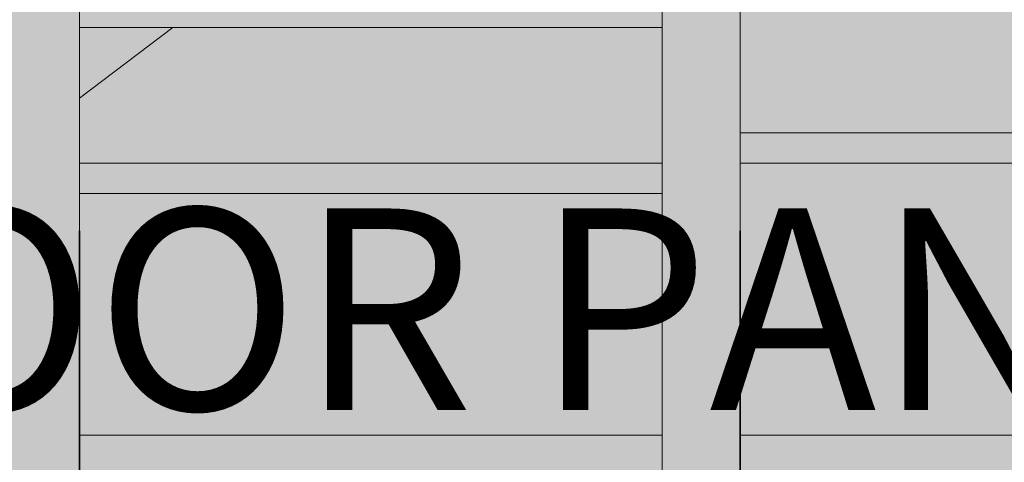
# Model space of a CAD drawing. Units: millimetres. Extents: x 130 to 1021, y 147 to 699.
# Tile 11 of 40: x 481 to 579, y 334 to 378. Entities that reach past the tile are written whole.
import ezdxf

# ---------------------------------------------------------------- set-up
doc = ezdxf.new("R2010")
doc.units = ezdxf.units.MM
doc.header["$MEASUREMENT"] = 0
for name, color, linetype, lineweight in [('A-ANNO-DIMS', 2, 'Continuous', 18), ('A-DOOR', 3, 'Continuous', 25), ('A-ELEV', 7, 'Continuous', 35), ('A-ELEV-PATT', 9, 'Continuous', 13), ('A-GLAZ', 4, 'Continuous', 18)]:
    doc.layers.add(name, color=color, linetype=linetype, lineweight=lineweight)
doc.styles.get("Standard").update_dxf_attribs({"font": 'arial.ttf'})
doc.dimstyles.get("Standard").update_dxf_attribs({"dimtxt": 20, "dimasz": 10, "dimexe": 10, "dimexo": 10, "dimgap": 5, "dimtad": 0, "dimtih": 1, "dimtoh": 1, "dimdec": 0, "dimzin": 0, "dimdsep": 46, "dimtxsty": 'Standard', "dimcen": 5, "dimadec": 0, "dimazin": 0, "dimtfac": 1, "dimtdec": 0, "dimtofl": 0, "dimtmove": 0, "dimatfit": 3, "dimfxl": 1, "dimtolj": 1, "dimtzin": 0, "dimarcsym": 0})

# ---------------------------------------------------------------- blocks, each defined once
blk = doc.blocks.new('*D7')
at = {"layer": 'A-ANNO-DIMS', "color": 0, "lineweight": -2, "transparency": 16777216}
for p, q in [((399.374, 349.447), (413.374, 349.447)), ((423.374, 349.447), (433.374, 349.447)), ((389.374, 344.547), (389.374, 339.447)), ((423.374, 344.547), (423.374, 339.447))]:
    blk.add_line(p, q, dxfattribs=at)
at = {"layer": 'A-ANNO-DIMS', "color": 0, "transparency": 16777216}
for points in [[(399.374, 351.114), (399.374, 347.781), (389.374, 349.447)], [(413.374, 351.114), (413.374, 347.781), (423.374, 349.447)]]:
    blk.add_solid(points, dxfattribs=at)
at = {"layer": 'Defpoints', "color": 0, "transparency": 16777216}
for p in [(389.374, 354.547), (423.374, 354.547), (423.374, 349.447)]:
    blk.add_point(p, dxfattribs=at)
at = {"layer": 'A-ANNO-DIMS', "color": 0, "transparency": 16777216, "insert": (582.037, 349.447), "char_height": 20, "attachment_point": 5}
blk.add_mtext('\\A1;DOOR PANEL 34 TYP.', dxfattribs=at)
blk = doc.blocks.new('*D8')
at = {"layer": 'A-ANNO-DIMS', "color": 0, "lineweight": -2, "transparency": 16777216}
for p, q in [((428.474, 380.947), (428.474, 390.947)), ((428.474, 390.947), (438.474, 390.947)), ((433.374, 370.947), (438.474, 370.947)), ((433.374, 354.547), (438.474, 354.547)), ((428.474, 344.547), (428.474, 334.547))]:
    blk.add_line(p, q, dxfattribs=at)
at = {"layer": 'A-ANNO-DIMS', "color": 0, "transparency": 16777216}
for points in [[(426.807, 380.947), (430.14, 380.947), (428.474, 370.947)], [(426.807, 344.547), (430.14, 344.547), (428.474, 354.547)]]:
    blk.add_solid(points, dxfattribs=at)
at = {"layer": 'Defpoints', "color": 0, "transparency": 16777216}
for p in [(423.374, 370.947), (428.474, 370.947), (423.374, 354.547)]:
    blk.add_point(p, dxfattribs=at)
at = {"layer": 'A-ANNO-DIMS', "color": 0, "transparency": 16777216, "insert": (491.209, 390.947), "char_height": 20, "attachment_point": 5}
blk.add_mtext('\\A1;16 TYP.', dxfattribs=at)
blk = doc.blocks.new('*D11')
at = {"layer": 'A-ANNO-DIMS', "color": 0, "lineweight": -2, "transparency": 16777216}
for p, q in [((737.374, 648.699), (737.374, 149.739)), ((299.374, 566.947), (299.374, 149.739)), ((309.374, 159.739), (490.857, 159.739)), ((727.374, 159.739), (545.891, 159.739))]:
    blk.add_line(p, q, dxfattribs=at)
at = {"layer": 'A-ANNO-DIMS', "color": 0, "transparency": 16777216}
for points in [[(309.374, 161.406), (309.374, 158.073), (299.374, 159.739)], [(727.374, 161.406), (727.374, 158.073), (737.374, 159.739)]]:
    blk.add_solid(points, dxfattribs=at)
at = {"layer": 'Defpoints', "color": 0, "transparency": 16777216}
for p in [(737.374, 658.699), (299.374, 576.947), (737.374, 159.739)]:
    blk.add_point(p, dxfattribs=at)
at = {"layer": 'A-ANNO-DIMS', "color": 0, "transparency": 16777216, "insert": (518.374, 159.739), "char_height": 20, "attachment_point": 5}
blk.add_mtext('\\A1;438', dxfattribs=at)
blk = doc.blocks.new('*D12')
at = {"layer": 'A-ANNO-DIMS', "color": 0, "lineweight": -2, "transparency": 16777216}
for p, q in [((477.374, 661.947), (265.074, 661.947)), ((275.074, 651.947), (275.074, 438.205)), ((275.074, 194.039), (275.074, 407.782)), ((357.163, 184.039), (265.074, 184.039))]:
    blk.add_line(p, q, dxfattribs=at)
at = {"layer": 'A-ANNO-DIMS', "color": 0, "transparency": 16777216}
for points in [[(273.407, 651.947), (276.74, 651.947), (275.074, 661.947)], [(273.407, 194.039), (276.74, 194.039), (275.074, 184.039)]]:
    blk.add_solid(points, dxfattribs=at)
at = {"layer": 'Defpoints', "color": 0, "transparency": 16777216}
for p in [(275.074, 661.947), (487.374, 661.947), (367.163, 184.039)]:
    blk.add_point(p, dxfattribs=at)
at = {"layer": 'A-ANNO-DIMS', "color": 0, "transparency": 16777216, "insert": (275.074, 422.993), "char_height": 20, "attachment_point": 5}
blk.add_mtext('\\A1;477.9', dxfattribs=at)
blk = doc.blocks.new('*D23')
at = {"layer": 'A-ANNO-DIMS', "color": 0, "lineweight": -2, "transparency": 16777216}
for p, q in [((466.767, 403.947), (466.767, 696.247)), ((475.988, 209.039), (475.988, 696.247)), ((456.767, 686.247), (446.767, 686.247)), ((485.988, 686.247), (495.988, 686.247))]:
    blk.add_line(p, q, dxfattribs=at)
at = {"layer": 'A-ANNO-DIMS', "color": 0, "transparency": 16777216}
for points in [[(456.767, 687.914), (456.767, 684.581), (466.767, 686.247)], [(485.988, 687.914), (485.988, 684.581), (475.988, 686.247)]]:
    blk.add_solid(points, dxfattribs=at)
at = {"layer": 'Defpoints', "color": 0, "transparency": 16777216}
for p in [(475.988, 686.247), (466.767, 393.947), (475.988, 199.039)]:
    blk.add_point(p, dxfattribs=at)
at = {"layer": 'A-ANNO-DIMS', "color": 0, "transparency": 16777216, "insert": (534.631, 686.247), "char_height": 20, "attachment_point": 5}
blk.add_mtext('\\A1;9.222', dxfattribs=at)
blk = doc.blocks.new('*D24')
at = {"layer": 'A-ANNO-DIMS', "color": 0, "lineweight": -2, "transparency": 16777216}
for p, q in [((475.988, 209.039), (475.988, 696.247)), ((487.374, 671.947), (487.374, 696.247)), ((465.988, 686.247), (455.988, 686.247)), ((497.374, 686.247), (507.374, 686.247))]:
    blk.add_line(p, q, dxfattribs=at)
at = {"layer": 'A-ANNO-DIMS', "color": 0, "transparency": 16777216}
for points in [[(465.988, 687.914), (465.988, 684.581), (475.988, 686.247)], [(497.374, 687.914), (497.374, 684.581), (487.374, 686.247)]]:
    blk.add_solid(points, dxfattribs=at)
at = {"layer": 'Defpoints', "color": 0, "transparency": 16777216}
for p in [(487.374, 686.247), (487.374, 661.947), (475.988, 199.039)]:
    blk.add_point(p, dxfattribs=at)
at = {"layer": 'A-ANNO-DIMS', "color": 0, "transparency": 16777216, "insert": (553.022, 686.247), "char_height": 20, "attachment_point": 5}
blk.add_mtext('\\A1;11.385', dxfattribs=at)
blk = doc.blocks.new('*D51')
at = {"layer": 'A-ANNO-DIMS', "color": 0, "lineweight": -2, "transparency": 16777216}
for p, q in [((554.635, 386.264), (771.674, 386.264)), ((761.674, 376.264), (761.674, 348.674)), ((761.674, 290.662), (761.674, 318.251)), ((554.635, 280.662), (771.674, 280.662))]:
    blk.add_line(p, q, dxfattribs=at)
at = {"layer": 'A-ANNO-DIMS', "color": 0, "transparency": 16777216}
for points in [[(760.007, 376.264), (763.34, 376.264), (761.674, 386.264)], [(760.007, 290.662), (763.34, 290.662), (761.674, 280.662)]]:
    blk.add_solid(points, dxfattribs=at)
at = {"layer": 'Defpoints', "color": 0, "transparency": 16777216}
for p in [(544.635, 386.264), (761.674, 386.264), (544.635, 280.662)]:
    blk.add_point(p, dxfattribs=at)
at = {"layer": 'A-ANNO-DIMS', "color": 0, "transparency": 16777216, "insert": (761.674, 333.463), "char_height": 20, "attachment_point": 5}
blk.add_mtext('\\A1;105.6', dxfattribs=at)
blk = doc.blocks.new('*D52')
at = {"layer": 'A-ANNO-DIMS', "color": 0, "lineweight": -2, "transparency": 16777216}
for p, q in [((761.674, 403.947), (761.674, 413.947)), ((761.674, 413.947), (771.674, 413.947)), ((642.818, 393.947), (771.674, 393.947)), ((554.635, 386.264), (771.674, 386.264)), ((761.674, 376.264), (761.674, 366.264))]:
    blk.add_line(p, q, dxfattribs=at)
at = {"layer": 'A-ANNO-DIMS', "color": 0, "transparency": 16777216}
for points in [[(760.007, 403.947), (763.34, 403.947), (761.674, 393.947)], [(760.007, 376.264), (763.34, 376.264), (761.674, 386.264)]]:
    blk.add_solid(points, dxfattribs=at)
at = {"layer": 'Defpoints', "color": 0, "transparency": 16777216}
for p in [(632.818, 393.947), (761.674, 393.947), (544.635, 386.264)]:
    blk.add_point(p, dxfattribs=at)
at = {"layer": 'A-ANNO-DIMS', "color": 0, "transparency": 16777216, "insert": (810.337, 413.947), "char_height": 20, "attachment_point": 5}
blk.add_mtext('\\A1;7.683', dxfattribs=at)
blk = doc.blocks.new('*D64')
at = {"layer": 'A-ANNO-DIMS', "color": 0, "lineweight": -2, "transparency": 16777216}
for p, q in [((502.049, 450.926), (502.049, 460.926)), ((497.049, 455.926), (507.049, 455.926)), ((363.96, 263.061), (409.922, 327.255)), ((353.96, 263.061), (363.96, 263.061))]:
    blk.add_line(p, q, dxfattribs=at)
at = {"layer": 'A-ANNO-DIMS', "color": 0, "transparency": 16777216}
blk.add_solid([(408.567, 328.225), (411.277, 326.284), (415.743, 335.385)], dxfattribs=at)
at = {"layer": 'Defpoints', "color": 0, "transparency": 16777216}
for p in [(502.049, 455.926), (415.743, 335.385)]:
    blk.add_point(p, dxfattribs=at)
at = {"layer": 'A-ANNO-DIMS', "color": 0, "transparency": 16777216, "insert": (297.8, 263.061), "char_height": 20, "attachment_point": 5}
blk.add_mtext('\\A1;R148.25', dxfattribs=at)
blk = doc.blocks.new('*D65')
at = {"layer": 'A-ANNO-DIMS', "color": 0, "lineweight": -2, "transparency": 16777216}
for p, q in [((495.463, 509.127), (472.508, 423.108)), ((505.463, 509.127), (495.463, 509.127)), ((427.374, 248.979), (427.374, 258.979)), ((422.374, 253.979), (432.374, 253.979))]:
    blk.add_line(p, q, dxfattribs=at)
at = {"layer": 'A-ANNO-DIMS', "color": 0, "transparency": 16777216}
blk.add_solid([(470.898, 423.538), (474.118, 422.679), (469.93, 413.447)], dxfattribs=at)
at = {"layer": 'Defpoints', "color": 0, "transparency": 16777216}
for p in [(469.93, 413.447), (427.374, 253.979)]:
    blk.add_point(p, dxfattribs=at)
at = {"layer": 'A-ANNO-DIMS', "color": 0, "transparency": 16777216, "insert": (561.623, 509.127), "char_height": 20, "attachment_point": 5}
blk.add_mtext('\\A1;R165.05', dxfattribs=at)
blk = doc.blocks.new('*D67')
at = {"layer": 'A-ANNO-DIMS', "color": 0, "lineweight": -2, "transparency": 16777216}
for p, q in [((479.756, 492.431), (462.144, 412.223)), ((489.756, 492.431), (479.756, 492.431)), ((427.07, 247.496), (427.07, 257.496)), ((422.07, 252.496), (432.07, 252.496))]:
    blk.add_line(p, q, dxfattribs=at)
at = {"layer": 'A-ANNO-DIMS', "color": 0, "transparency": 16777216}
blk.add_solid([(460.516, 412.58), (463.772, 411.865), (459.999, 402.455)], dxfattribs=at)
at = {"layer": 'Defpoints', "color": 0, "transparency": 16777216}
for p in [(459.999, 402.455), (427.07, 252.496)]:
    blk.add_point(p, dxfattribs=at)
at = {"layer": 'A-ANNO-DIMS', "color": 0, "transparency": 16777216, "insert": (545.841, 492.431), "char_height": 20, "attachment_point": 5}
blk.add_mtext('\\A1;R153.53', dxfattribs=at)
blk = doc.blocks.new('*D69')
at = {"layer": 'A-ANNO-DIMS', "color": 0, "lineweight": -2, "transparency": 16777216}
for p, q in [((507.746, 572.261), (483.091, 501.813)), ((517.746, 572.261), (507.746, 572.261)), ((433.191, 354.23), (433.191, 364.23)), ((428.191, 359.23), (438.191, 359.23))]:
    blk.add_line(p, q, dxfattribs=at)
at = {"layer": 'A-ANNO-DIMS', "color": 0, "transparency": 16777216}
blk.add_solid([(481.518, 502.363), (484.664, 501.262), (479.788, 492.374)], dxfattribs=at)
at = {"layer": 'Defpoints', "color": 0, "transparency": 16777216}
for p in [(479.788, 492.374), (433.191, 359.23)]:
    blk.add_point(p, dxfattribs=at)
at = {"layer": 'A-ANNO-DIMS', "color": 0, "transparency": 16777216, "insert": (573.824, 572.261), "char_height": 20, "attachment_point": 5}
blk.add_mtext('\\A1;R141.06', dxfattribs=at)
blk = doc.blocks.new('*D71')
at = {"layer": 'A-ANNO-DIMS', "color": 0, "lineweight": -2, "transparency": 16777216}
for p, q in [((492.108, 581.609), (472.542, 512.666)), ((502.108, 581.609), (492.108, 581.609)), ((432.65, 367.109), (432.65, 377.109)), ((427.65, 372.109), (437.65, 372.109))]:
    blk.add_line(p, q, dxfattribs=at)
at = {"layer": 'A-ANNO-DIMS', "color": 0, "transparency": 16777216}
blk.add_solid([(470.938, 513.121), (474.145, 512.211), (469.812, 503.046)], dxfattribs=at)
at = {"layer": 'Defpoints', "color": 0, "transparency": 16777216}
for p in [(469.812, 503.046), (432.65, 372.109)]:
    blk.add_point(p, dxfattribs=at)
at = {"layer": 'A-ANNO-DIMS', "color": 0, "transparency": 16777216, "insert": (548.493, 581.609), "char_height": 20, "attachment_point": 5}
blk.add_mtext('\\A1;R136.1', dxfattribs=at)
blk = doc.blocks.new('*D72')
at = {"layer": 'A-ANNO-DIMS', "color": 0, "lineweight": -2, "transparency": 16777216}
for p, q in [((460.658, 573.64), (451.279, 503.49)), ((470.658, 573.64), (460.658, 573.64)), ((432.115, 355.142), (432.115, 365.142)), ((427.115, 360.142), (437.115, 360.142))]:
    blk.add_line(p, q, dxfattribs=at)
at = {"layer": 'A-ANNO-DIMS', "color": 0, "transparency": 16777216}
blk.add_solid([(449.628, 503.711), (452.931, 503.27), (449.954, 493.579)], dxfattribs=at)
at = {"layer": 'Defpoints', "color": 0, "transparency": 16777216}
for p in [(449.954, 493.579), (432.115, 360.142)]:
    blk.add_point(p, dxfattribs=at)
at = {"layer": 'A-ANNO-DIMS', "color": 0, "transparency": 16777216, "insert": (526.64, 573.64), "char_height": 20, "attachment_point": 5}
blk.add_mtext('\\A1;R134.62', dxfattribs=at)

msp = doc.modelspace()

# ---------------------------------------------------------------- hatches: boundary and pattern name
at = {"layer": 'A-ELEV-PATT'}
h = msp.add_hatch(color=256, dxfattribs=at)
h.dxf.hatch_style = 1
h.paths.add_polyline_path([(737.3738, 658.6988, 0.0135961), (632.4019, 661.9473), (607.3738, 661.9473), (487.3738, 661.9473), (487.3738, 649.9473), (607.3738, 649.9473), (632.3794, 649.9473, -0.0136841), (737.3738, 646.6784)])
h.paths.add_polyline_path([(732.3738, 643.9599, 0.0130529), (632.3738, 646.9473), (607.3738, 646.9473), (487.3738, 646.9473), (487.3738, 596.9473), (632.3738, 596.9473, -0.0130529), (732.3738, 593.9599)])
h.paths.add_polyline_path([(737.3738, 593.6732, 0.0137063), (632.3738, 596.9473), (487.3738, 596.9473), (487.3738, 586.9473), (632.355, 586.9473, -0.0137808), (737.3738, 583.6559)])
h.paths.add_polyline_path([(447.3738, 646.9473), (307.3738, 646.9473), (302.3738, 646.9473), (302.3738, 634.9473), (447.3738, 634.9473)])
h.paths.add_polyline_path([(447.3738, 631.9473), (307.3738, 631.9473), (307.3738, 586.9473), (447.3738, 586.9473)])
h.paths.add_polyline_path([(447.3738, 586.9473), (307.3738, 586.9473), (302.3738, 586.9473), (302.3738, 576.9473), (447.3738, 576.9473)])
h.paths.add_polyline_path([(447.3738, 573.9473), (367.3738, 573.9473), (367.3738, 539.9473), (447.3738, 539.9473)])
h.paths.add_polyline_path([(447.3738, 537.9473), (367.3738, 537.9473), (367.3738, 507.9473), (400.392, 507.4253, -0.001728), (401.3281, 507.6451, -0.5220025), (425.6117, 511.0391, -0.0391849), (447.3738, 510.4359), (447.3738, 510.7883)])
h.paths.add_polyline_path([(394.7238, 505.9473), (367.3738, 505.9473), (367.3738, 476.9473, -0.0146512), (375.8501, 480.2159), (376.1506, 499.2266, -0.0355419)])
h.paths.add_polyline_path([(632.3738, 583.9473), (552.3738, 583.9473), (552.3738, 550.9473), (632.3738, 550.9473)])
h.paths.add_polyline_path([(632.3738, 548.9473), (552.3738, 548.9473), (552.3738, 515.9473), (632.3738, 515.9473)])
h.paths.add_polyline_path([(632.3738, 513.9473), (552.3738, 513.9473), (552.3738, 476.9473), (632.3738, 476.9473)])
h.paths.add_polyline_path([(737.3738, 473.6903, 0.0136326), (632.3926, 476.9473), (552.3738, 476.9473), (487.3738, 476.9473), (487.3738, 466.9473), (632.3738, 466.9473, -0.0137063), (737.3738, 463.6732)])
h.paths.add_polyline_path([(732.3738, 460.9552, 0.0130741), (632.3681, 463.9473), (487.3738, 463.9473), (487.3738, 407.735, -0.0032286), (489.3544, 406.9473), (632.3926, 406.9473, -0.0129826), (732.3738, 403.9755)])
h.paths.add_polyline_path([(487.3738, 463.9473, 0.20133), (367.3738, 463.9473), (367.3738, 407.735, -0.1882031), (487.3738, 407.735)])
h.paths.add_polyline_path([(367.3738, 476.9473), (367.3738, 466.9473, -0.2013309), (487.3738, 466.9473), (487.3738, 476.9473, 0.20133)])
h.paths.add_polyline_path([(367.3738, 463.9473), (307.3738, 463.9473), (307.3738, 401.9473), (357.9413, 401.9473), (367.3738, 407.735)])
h.paths.add_polyline_path([(367.3738, 476.9473), (302.3738, 476.9473), (302.3738, 466.9473), (367.3738, 466.9473)])
h.paths.add_polyline_path([(632.8184, 366.9453), (552.3738, 366.9453), (552.3738, 393.9473), (632.8184, 393.9473)])
h.paths.add_polyline_path([(632.8184, 357.2114), (632.8184, 363.9453), (552.3738, 363.9453), (552.3738, 357.2114), (552.3738, 336.9453), (632.8184, 336.9453)])
h.paths.add_polyline_path([(632.8184, 333.9453), (552.3738, 333.9453), (552.3738, 306.9453), (632.8184, 306.9453)])
h.paths.add_polyline_path([(632.8184, 303.9453), (552.3738, 303.9453), (552.3738, 273.9473), (632.355, 273.9473, 0.0000608), (632.8184, 273.9491)])
h.paths.add_polyline_path([(737.3738, 403.6903, 0.0136326), (632.3926, 406.9473), (489.3544, 406.9473, 0.1915481), (367.3738, 407.735), (367.3738, 396.9473, -0.2013309), (487.3738, 396.9473), (632.3738, 396.9473, -0.0137063), (737.3738, 393.6732)])
h.paths.add_polyline_path([(357.9413, 401.9473), (307.3738, 401.9473), (307.3738, 391.9473), (357.9413, 391.9473)])
h.paths.add_polyline_path([(357.9413, 357.2114), (357.9413, 388.9473), (307.3738, 388.9473), (307.3738, 357.2114), (307.3738, 273.9473), (357.9413, 273.9473)])
h.paths.add_polyline_path([(732.3738, 263.93, -0.0130317), (632.3794, 260.9473), (466.7667, 260.9473), (466.7667, 240.9473), (469.8406, 236.978), (469.8406, 221.978), (472.9145, 218.0087), (472.9145, 213.9473), (607.3738, 213.9473), (732.3738, 213.9473)])
h.paths.add_polyline_path([(732.3738, 290.889), (722.479, 290.889), (722.479, 301.889), (732.3738, 301.889), (732.3738, 305.889), (722.479, 305.889), (722.479, 316.889), (732.3738, 316.889), (732.3738, 320.889), (722.479, 320.889), (722.479, 331.889), (732.3738, 331.889), (732.3738, 335.889), (722.479, 335.889), (722.479, 346.889), (732.3738, 346.889), (732.3738, 350.889), (722.479, 350.889), (722.479, 361.889), (732.3738, 361.889), (732.3738, 365.889), (722.479, 365.889), (722.479, 376.889), (732.3738, 376.889), (732.3738, 380.889), (722.479, 380.889), (722.479, 391.4848, 0.0005233), (718.479, 391.6843), (718.479, 380.889), (707.479, 380.889), (707.479, 392.1896, 0.0005231), (703.479, 392.3576), (703.479, 380.889), (692.479, 380.889), (692.479, 392.7765, 0.0005229), (688.479, 392.9131), (688.479, 380.889), (677.479, 380.889), (677.479, 393.2456, 0.0005228), (673.479, 393.3508), (673.479, 380.889), (662.479, 380.889), (662.479, 393.597, 0.0005227), (658.479, 393.6709), (658.479, 380.889), (647.479, 380.889), (647.479, 393.8308, 0.0005226), (643.479, 393.8732), (643.479, 380.889), (632.8184, 380.889), (632.8184, 376.889), (643.479, 376.889), (643.479, 365.889), (632.8184, 365.889), (632.8184, 361.889), (643.479, 361.889), (643.479, 350.889), (632.8184, 350.889), (632.8184, 346.889), (643.479, 346.889), (643.479, 335.889), (632.8184, 335.889), (632.8184, 331.889), (643.479, 331.889), (643.479, 320.889), (632.8184, 320.889), (632.8184, 316.889), (643.479, 316.889), (643.479, 305.889), (632.8184, 305.889), (632.8184, 301.889), (643.479, 301.889), (643.479, 290.889), (632.8184, 290.889), (632.8184, 286.889), (643.479, 286.889), (643.479, 274.0217, 0.0005246), (647.479, 274.0643), (647.479, 286.889), (658.479, 286.889), (658.479, 274.2248, 0.0005246), (662.479, 274.2989), (662.479, 286.889), (673.479, 286.889), (673.479, 274.546, 0.0005247), (677.479, 274.6516), (677.479, 286.889), (688.479, 286.889), (688.479, 274.9853, 0.0005248), (692.479, 275.1224), (692.479, 286.889), (703.479, 286.889), (703.479, 275.5429, 0.000525), (707.479, 275.7115), (707.479, 286.889), (718.479, 286.889), (718.479, 276.2187, 0.0005252), (722.479, 276.4189), (722.479, 286.889), (732.3738, 286.889)])
h.paths.add_polyline_path([(718.479, 290.889), (707.479, 290.889), (707.479, 301.889), (718.479, 301.889)], flags=16)
h.paths.add_polyline_path([(703.479, 290.889), (692.479, 290.889), (692.479, 301.889), (703.479, 301.889)], flags=16)
h.paths.add_polyline_path([(718.479, 305.889), (707.479, 305.889), (707.479, 316.889), (718.479, 316.889)], flags=16)
h.paths.add_polyline_path([(703.479, 305.889), (692.479, 305.889), (692.479, 316.889), (703.479, 316.889)], flags=16)
h.paths.add_polyline_path([(688.479, 290.889), (677.479, 290.889), (677.479, 301.889), (688.479, 301.889)], flags=16)
h.paths.add_polyline_path([(718.479, 320.889), (707.479, 320.889), (707.479, 331.889), (718.479, 331.889)], flags=16)
h.paths.add_polyline_path([(688.479, 305.889), (677.479, 305.889), (677.479, 316.889), (688.479, 316.889)], flags=16)
h.paths.add_polyline_path([(703.479, 320.889), (692.479, 320.889), (692.479, 331.889), (703.479, 331.889)], flags=16)
h.paths.add_polyline_path([(688.479, 320.889), (677.479, 320.889), (677.479, 331.889), (688.479, 331.889)], flags=16)
h.paths.add_polyline_path([(673.479, 290.889), (662.479, 290.889), (662.479, 301.889), (673.479, 301.889)], flags=16)
h.paths.add_polyline_path([(718.479, 335.889), (707.479, 335.889), (707.479, 346.889), (718.479, 346.889)], flags=16)
h.paths.add_polyline_path([(673.479, 305.889), (662.479, 305.889), (662.479, 316.889), (673.479, 316.889)], flags=16)
h.paths.add_polyline_path([(703.479, 335.889), (692.479, 335.889), (692.479, 346.889), (703.479, 346.889)], flags=16)
h.paths.add_polyline_path([(673.479, 320.889), (662.479, 320.889), (662.479, 331.889), (673.479, 331.889)], flags=16)
h.paths.add_polyline_path([(688.479, 335.889), (677.479, 335.889), (677.479, 346.889), (688.479, 346.889)], flags=16)
h.paths.add_polyline_path([(658.479, 290.889), (647.479, 290.889), (647.479, 301.889), (658.479, 301.889)], flags=16)
h.paths.add_polyline_path([(718.479, 350.889), (707.479, 350.889), (707.479, 361.889), (718.479, 361.889)], flags=16)
h.paths.add_polyline_path([(658.479, 305.889), (647.479, 305.889), (647.479, 316.889), (658.479, 316.889)], flags=16)
h.paths.add_polyline_path([(703.479, 350.889), (692.479, 350.889), (692.479, 361.889), (703.479, 361.889)], flags=16)
h.paths.add_polyline_path([(673.479, 335.889), (662.479, 335.889), (662.479, 346.889), (673.479, 346.889)], flags=16)
h.paths.add_polyline_path([(658.479, 320.889), (647.479, 320.889), (647.479, 331.889), (658.479, 331.889)], flags=16)
h.paths.add_polyline_path([(688.479, 350.889), (677.479, 350.889), (677.479, 361.889), (688.479, 361.889)], flags=16)
h.paths.add_polyline_path([(718.479, 365.889), (707.479, 365.889), (707.479, 376.889), (718.479, 376.889)], flags=16)
h.paths.add_polyline_path([(658.479, 335.889), (647.479, 335.889), (647.479, 346.889), (658.479, 346.889)], flags=16)
h.paths.add_polyline_path([(673.479, 350.889), (662.479, 350.889), (662.479, 361.889), (673.479, 361.889)], flags=16)
h.paths.add_polyline_path([(703.479, 365.889), (692.479, 365.889), (692.479, 376.889), (703.479, 376.889)], flags=16)
h.paths.add_polyline_path([(688.479, 365.889), (677.479, 365.889), (677.479, 376.889), (688.479, 376.889)], flags=16)
h.paths.add_polyline_path([(658.479, 350.889), (647.479, 350.889), (647.479, 361.889), (658.479, 361.889)], flags=16)
h.paths.add_polyline_path([(673.479, 365.889), (662.479, 365.889), (662.479, 376.889), (673.479, 376.889)], flags=16)
h.paths.add_polyline_path([(658.479, 365.889), (647.479, 365.889), (647.479, 376.889), (658.479, 376.889)], flags=16)
h.paths.add_polyline_path([(732.3738, 503.9786), (722.3392, 503.9786), (722.3392, 514.9786), (732.3738, 514.9786), (732.3738, 518.9786), (722.3392, 518.9786), (722.3392, 529.9786), (732.3738, 529.9786), (732.3738, 533.9786), (722.3392, 533.9786), (722.3392, 544.9786), (732.3738, 544.9786), (732.3738, 546.9473), (732.3738, 548.9786), (722.3392, 548.9786), (722.3392, 559.9786), (732.3738, 559.9786), (732.3738, 563.9786), (722.3392, 563.9786), (722.3392, 574.9786), (732.3738, 574.9786), (732.3738, 578.9786), (722.3392, 578.9786), (722.3392, 581.4789, 0.000526), (718.3392, 581.6791), (718.3392, 578.9786), (707.3392, 578.9786), (707.3392, 582.1863, 0.0005258), (703.3392, 582.355), (703.3392, 578.9786), (692.3392, 578.9786), (692.3392, 582.7752, 0.0005257), (688.3392, 582.9123), (688.3392, 578.9786), (677.3392, 578.9786), (677.3392, 583.2457, 0.0005255), (673.3392, 583.3512), (673.3392, 578.9786), (662.3392, 578.9786), (662.3392, 583.5978, 0.0005254), (658.3392, 583.6718), (658.3392, 578.9786), (647.3392, 578.9786), (647.3392, 583.8317, 0.0005254), (643.3392, 583.8741), (643.3392, 578.9786), (632.3738, 578.9786), (632.3738, 574.9786), (643.3392, 574.9786), (643.3392, 563.9786), (632.3738, 563.9786), (632.3738, 559.9786), (643.3392, 559.9786), (643.3392, 548.9786), (632.3738, 548.9786), (632.3738, 544.9786), (643.3392, 544.9786), (643.3392, 533.9786), (632.3738, 533.9786), (632.3738, 529.9786), (643.3392, 529.9786), (643.3392, 518.9786), (632.3738, 518.9786), (632.3738, 515.9473), (632.3738, 514.9786), (643.3392, 514.9786), (643.3392, 503.9786), (632.3738, 503.9786), (632.3738, 499.9786), (643.3392, 499.9786), (643.3392, 488.9786), (632.3738, 488.9786), (632.3738, 484.9786), (643.3392, 484.9786), (643.3392, 476.8751, -0.0005191), (647.3392, 476.8332), (647.3392, 484.9786), (658.3392, 484.9786), (658.3392, 476.6752, -0.0005192), (662.3392, 476.6022), (662.3392, 484.9786), (673.3392, 484.9786), (673.3392, 476.3585, -0.0005193), (677.3392, 476.2543), (677.3392, 484.9786), (688.3392, 484.9786), (688.3392, 475.9248, -0.0005194), (692.3392, 475.7894), (692.3392, 484.9786), (703.3392, 484.9786), (703.3392, 475.3741, -0.0005195), (707.3392, 475.2075), (707.3392, 484.9786), (718.3392, 484.9786), (718.3392, 474.7064, -0.0005197), (722.3392, 474.5086), (722.3392, 484.9786), (732.3738, 484.9786), (732.3738, 488.9786), (722.3392, 488.9786), (722.3392, 499.9786), (732.3738, 499.9786)])
h.paths.add_polyline_path([(718.3392, 503.9786), (707.3392, 503.9786), (707.3392, 514.9786), (718.3392, 514.9786)], flags=16)
h.paths.add_polyline_path([(718.3392, 499.9786), (718.3392, 488.9786), (707.3392, 488.9786), (707.3392, 499.9786)], flags=16)
h.paths.add_polyline_path([(718.3392, 518.9786), (707.3392, 518.9786), (707.3392, 529.9786), (718.3392, 529.9786)], flags=16)
h.paths.add_polyline_path([(703.3392, 503.9786), (692.3392, 503.9786), (692.3392, 514.9786), (703.3392, 514.9786)], flags=16)
h.paths.add_polyline_path([(703.3392, 499.9786), (703.3392, 488.9786), (692.3392, 488.9786), (692.3392, 499.9786)], flags=16)
h.paths.add_polyline_path([(703.3392, 518.9786), (692.3392, 518.9786), (692.3392, 529.9786), (703.3392, 529.9786)], flags=16)
h.paths.add_polyline_path([(718.3392, 533.9786), (707.3392, 533.9786), (707.3392, 544.9786), (718.3392, 544.9786)], flags=16)
h.paths.add_polyline_path([(688.3392, 503.9786), (677.3392, 503.9786), (677.3392, 514.9786), (688.3392, 514.9786)], flags=16)
h.paths.add_polyline_path([(688.3392, 499.9786), (688.3392, 488.9786), (677.3392, 488.9786), (677.3392, 499.9786)], flags=16)
h.paths.add_polyline_path([(703.3392, 533.9786), (692.3392, 533.9786), (692.3392, 544.9786), (703.3392, 544.9786)], flags=16)
h.paths.add_polyline_path([(688.3392, 518.9786), (677.3392, 518.9786), (677.3392, 529.9786), (688.3392, 529.9786)], flags=16)
h.paths.add_polyline_path([(688.3392, 533.9786), (677.3392, 533.9786), (677.3392, 544.9786), (688.3392, 544.9786)], flags=16)
h.paths.add_polyline_path([(718.3392, 548.9786), (707.3392, 548.9786), (707.3392, 559.9786), (718.3392, 559.9786)], flags=16)
h.paths.add_polyline_path([(673.3392, 503.9786), (662.3392, 503.9786), (662.3392, 514.9786), (673.3392, 514.9786)], flags=16)
h.paths.add_polyline_path([(673.3392, 499.9786), (673.3392, 488.9786), (662.3392, 488.9786), (662.3392, 499.9786)], flags=16)
h.paths.add_polyline_path([(703.3392, 548.9786), (692.3392, 548.9786), (692.3392, 559.9786), (703.3392, 559.9786)], flags=16)
h.paths.add_polyline_path([(673.3392, 518.9786), (662.3392, 518.9786), (662.3392, 529.9786), (673.3392, 529.9786)], flags=16)
h.paths.add_polyline_path([(688.3392, 548.9786), (677.3392, 548.9786), (677.3392, 559.9786), (688.3392, 559.9786)], flags=16)
h.paths.add_polyline_path([(673.3392, 533.9786), (662.3392, 533.9786), (662.3392, 544.9786), (673.3392, 544.9786)], flags=16)
h.paths.add_polyline_path([(718.3392, 563.9786), (707.3392, 563.9786), (707.3392, 574.9786), (718.3392, 574.9786)], flags=16)
h.paths.add_polyline_path([(658.3392, 503.9786), (647.3392, 503.9786), (647.3392, 514.9786), (658.3392, 514.9786)], flags=16)
h.paths.add_polyline_path([(658.3392, 499.9786), (658.3392, 488.9786), (647.3392, 488.9786), (647.3392, 499.9786)], flags=16)
h.paths.add_polyline_path([(703.3392, 563.9786), (692.3392, 563.9786), (692.3392, 574.9786), (703.3392, 574.9786)], flags=16)
h.paths.add_polyline_path([(658.3392, 518.9786), (647.3392, 518.9786), (647.3392, 529.9786), (658.3392, 529.9786)], flags=16)
h.paths.add_polyline_path([(673.3392, 548.9786), (662.3392, 548.9786), (662.3392, 559.9786), (673.3392, 559.9786)], flags=16)
h.paths.add_polyline_path([(688.3392, 563.9786), (677.3392, 563.9786), (677.3392, 574.9786), (688.3392, 574.9786)], flags=16)
h.paths.add_polyline_path([(658.3392, 533.9786), (647.3392, 533.9786), (647.3392, 544.9786), (658.3392, 544.9786)], flags=16)
h.paths.add_polyline_path([(673.3392, 563.9786), (662.3392, 563.9786), (662.3392, 574.9786), (673.3392, 574.9786)], flags=16)
h.paths.add_polyline_path([(658.3392, 548.9786), (647.3392, 548.9786), (647.3392, 559.9786), (658.3392, 559.9786)], flags=16)
h.paths.add_polyline_path([(658.3392, 563.9786), (647.3392, 563.9786), (647.3392, 574.9786), (658.3392, 574.9786)], flags=16)
h = msp.add_hatch(color=256, dxfattribs=at)
h.paths.add_polyline_path([(327.3738, 569.884), (327.3738, 573.9473), (307.3738, 573.9473), (307.3738, 476.9473), (327.3738, 476.9473), (327.3738, 480.95)])
h.paths.add_polyline_path([(486.7667, 386.2639), (486.7667, 393.9473), (466.7667, 393.9473), (466.7667, 357.2114), (466.7667, 311.9335, 0.0342703), (486.7667, 308.4637)])
h.paths.add_polyline_path([(486.7667, 308.4637, -0.0342703), (466.7667, 311.9335), (466.7667, 273.9473), (486.7667, 273.9473)])
h.paths.add_polyline_path([(389.3738, 351.5473), (396.7693, 351.5473, -0.007027), (393.8774, 354.5473), (389.3738, 354.5473), (389.3738, 359.5775, -0.0190302), (382.3738, 368.424), (382.3738, 249.5473), (432.3738, 249.5473), (432.3738, 325.067, -0.0057673), (429.3738, 326.709), (429.3738, 257.5473), (426.3738, 257.5473), (426.3738, 328.4428, -0.0059254), (423.3738, 330.272), (423.3738, 315.7473), (389.3738, 315.7473), (389.3738, 332.1473), (420.4552, 332.1473, -0.008951), (416.0768, 335.1473), (389.3738, 335.1473)])
h.paths.add_polyline_path([(389.3738, 312.7473), (423.3738, 312.7473), (423.3738, 296.3473), (389.3738, 296.3473)], flags=16)
h.paths.add_polyline_path([(389.3738, 293.3473), (423.3738, 293.3473), (423.3738, 276.9473), (389.3738, 276.9473)], flags=16)
h.paths.add_polyline_path([(389.3738, 273.9473), (423.3738, 273.9473), (423.3738, 257.5473), (389.3738, 257.5473)], flags=16)
h.paths.add_polyline_path([(432.3738, 378.9473), (382.3738, 378.9473), (382.3738, 368.424, 0.0190302), (389.3738, 359.5775), (389.3738, 370.9473), (423.3738, 370.9473), (423.3738, 354.5473), (393.8774, 354.5473, 0.007027), (396.7693, 351.5473), (423.3738, 351.5473), (423.3738, 335.1473), (416.0768, 335.1473, 0.008951), (420.4552, 332.1473), (423.3738, 332.1473), (423.3738, 330.272, 0.0059254), (426.3738, 328.4428), (426.3738, 370.9473), (429.3738, 370.9473), (429.3738, 326.709, 0.0057673), (432.3738, 325.067)])
h.paths.add_polyline_path([(466.7667, 357.2114), (466.7667, 393.9473), (447.3738, 393.9473), (447.3738, 357.2114), (447.3738, 318.1243, 0.0063261), (450.8779, 316.785), (450.8779, 331.5915), (463.5608, 331.5915), (463.5608, 312.7571, 0.005582), (466.7667, 311.9335)])
h.paths.add_polyline_path([(450.8779, 334.5915), (450.8779, 360.0915), (463.5608, 360.0915), (463.5608, 334.5915)], flags=16)
h.paths.add_polyline_path([(450.8779, 363.0915), (450.8779, 388.6449), (463.5608, 388.6449), (463.5608, 363.0915)], flags=16)
h.paths.add_polyline_path([(466.7667, 311.9335, -0.005582), (463.5608, 312.7571), (463.5608, 306.0915), (450.8779, 306.0915), (450.8779, 316.785, -0.0063261), (447.3738, 318.1243), (447.3738, 273.9473), (466.7667, 273.9473)])
h.paths.add_polyline_path([(450.8779, 303.0915), (463.5608, 303.0915), (463.5608, 277.5915), (450.8779, 277.5915)], flags=16)
h.paths.add_polyline_path([(552.3738, 357.2114), (552.3738, 393.9473), (486.7667, 393.9473), (486.7667, 386.2639), (544.6354, 386.2639), (544.6354, 280.6619), (486.7667, 280.6619), (486.7667, 273.9473), (552.3738, 273.9473)])
h.paths.add_polyline_path([(487.3738, 583.9473), (472.3738, 580.1973), (472.3738, 507.0765), (472.3738, 505.4251, -0.0056452), (475.3738, 504.4942), (475.3738, 506.3543), (475.3738, 511.9473), (484.3738, 511.9473), (484.3738, 503.8134), (484.3738, 501.2439, -0.0058357), (487.3738, 500.0015)])
h.paths.add_polyline_path([(484.3738, 578.0434), (484.3738, 548.9473), (475.3738, 548.9473), (475.3738, 575.7934)], flags=16)
h.paths.add_polyline_path([(484.3738, 546.9473), (484.3738, 513.9473), (475.3738, 513.9473), (475.3738, 518.7148), (475.3738, 546.9473)], flags=16)
h = msp.add_hatch(color=256, dxfattribs=at)
h.dxf.hatch_style = 1
h.paths.add_polyline_path([(363.922, 569.884), (327.3738, 569.884), (327.3738, 557.9168), (363.922, 557.9168)])
h.paths.add_polyline_path([(547.7773, 577.3739), (502.3738, 577.3739), (502.3738, 566.2111), (547.7773, 566.2111)])
h.paths.add_polyline_path([(544.6354, 386.2639), (486.7667, 386.2639), (486.7667, 377.43), (544.6354, 377.43)])
h.paths.add_polyline_path([(496.0546, 377.43), (486.7667, 377.43), (486.7667, 370.4028)])
h.paths.add_polyline_path([(447.3738, 393.9473), (367.3738, 393.9473, 0.0500478), (382.3738, 368.424), (382.3738, 378.9473), (432.3738, 378.9473), (432.3738, 325.067, 0.0278945), (447.3738, 318.1243), (447.3738, 357.2114)])
h.paths.add_polyline_path([(463.5608, 388.6449), (450.8779, 388.6449), (450.8779, 363.0915), (463.5608, 363.0915)])
h.paths.add_polyline_path([(463.5608, 360.0915), (450.8779, 360.0915), (450.8779, 334.5915), (463.5608, 334.5915)])
h.paths.add_polyline_path([(463.5608, 331.5915), (450.8779, 331.5915), (450.8779, 316.785, 0.0224513), (463.5608, 312.7571)])
h = msp.add_hatch(color=256, dxfattribs=at)
h.dxf.hatch_style = 1
h.paths.add_polyline_path([(502.3738, 566.2111), (502.3738, 548.9473), (547.7773, 548.9473), (547.7773, 566.2111)])
h.paths.add_polyline_path([(502.3738, 546.9473), (502.3738, 537.2685), (547.7773, 537.2685), (547.7773, 546.9473)])
h.paths.add_polyline_path([(486.7667, 360.9454), (486.7667, 336.9454), (544.6354, 336.9453), (544.6354, 360.9453)])
h.paths.add_polyline_path([(496.0546, 377.43), (486.7667, 370.4028), (486.7667, 363.9454), (544.6354, 363.9453), (544.6354, 377.43)])
h = msp.add_hatch(color=256, dxfattribs=at)
h.dxf.hatch_style = 1
h.paths.add_polyline_path([(447.3738, 537.9473), (447.3738, 539.9473), (367.3738, 539.9473), (367.3738, 537.9473)])
h.paths.add_polyline_path([(394.7238, 505.9473, -0.0105284), (400.392, 507.4253), (367.3738, 507.9473), (367.3738, 505.9473)])
h.paths.add_polyline_path([(547.7773, 546.9473), (547.7773, 548.9473), (502.3738, 548.9473), (502.3738, 546.9473)])
h.paths.add_polyline_path([(632.3738, 548.9473), (632.3738, 550.9473), (552.3738, 550.9473), (552.3738, 548.9473)])
h.paths.add_polyline_path([(632.3738, 513.9473), (632.3738, 515.9473), (552.3738, 515.9473), (552.3738, 513.9473)])
h.paths.add_polyline_path([(544.6354, 360.9453), (544.6354, 363.9453), (486.7667, 363.9454), (486.7667, 360.9454)])
h.paths.add_polyline_path([(632.8184, 363.9453), (632.8184, 366.9453), (552.3738, 366.9453), (552.3738, 363.9453)])
h.paths.add_polyline_path([(632.8184, 333.9453), (632.8184, 336.9453), (552.3738, 336.9453), (552.3738, 333.9453)])
h.paths.add_polyline_path([(552.3738, 306.9453), (552.3738, 303.9453), (632.8184, 303.9453), (632.8184, 306.9453)])
msp.add_hatch(color=256, dxfattribs=at).paths.add_polyline_path([(486.7667, 336.9454), (486.7667, 333.4629), (544.6354, 333.4629), (544.6354, 336.9453)])

# ---------------------------------------------------------------- linework, layer by layer
at = {"layer": 'A-DOOR'}
msp.add_arc((502.0489, 455.9263), 148.2524, 204.712441, 264.083334, dxfattribs=at)
at = {"layer": 'A-ELEV'}
for p, q in [((486.7667, 357.2114), (486.7667, 273.9473)), ((552.3738, 357.2114), (552.3738, 273.9473))]:
    msp.add_line(p, q, dxfattribs=at)
at = {"layer": 'A-GLAZ'}
for p, q in [((486.7667, 393.9473), (486.7667, 357.2114)), ((552.3738, 393.9473), (552.3738, 357.2114)), ((544.6354, 377.43), (486.7667, 377.43)), ((486.7667, 370.4028), (496.0546, 377.43)), ((552.3738, 366.9453), (632.8184, 366.9453)), ((486.7667, 363.9454), (544.6354, 363.9453)), ((552.3738, 363.9453), (632.8184, 363.9453)), ((486.7667, 360.9454), (544.6354, 360.9453)), ((486.7667, 336.9454), (544.6354, 336.9453)), ((552.3738, 336.9453), (632.8184, 336.9453))]:
    msp.add_line(p, q, dxfattribs=at)
msp.add_lwpolyline([(544.6354, 386.2639), (486.7667, 386.2639), (486.7667, 280.6619), (544.6354, 280.6619)], close=True, dxfattribs=at)

# ---------------------------------------------------------------- dimensions: what is measured, and where the dimension line sits
at = {"layer": 'A-ANNO-DIMS'}
for base, p1, p2, override, picture, middle in [((475.9885, 686.2473), (466.7667, 393.9473), (475.9885, 199.0395), {"dimdec": 3, "dimlfac": 1, "dimrnd": 0, "dimzin": 0, "dimdsep": 46, "dimlunit": 2}, '*D23', (534.631, 686.2473)), ((487.3738, 686.2473), (475.9885, 199.0395), (487.3738, 661.9473), {"dimdec": 3, "dimlfac": 1, "dimrnd": 0, "dimzin": 0, "dimdsep": 46, "dimlunit": 2}, '*D24', (553.0218, 686.2473)), ((737.3738, 159.7395), (299.3738, 576.9473), (737.3738, 658.6988), {"dimdec": 0, "dimlfac": 1, "dimrnd": 0, "dimzin": 0, "dimdsep": 46, "dimlunit": 2}, '*D11', (518.3738, 159.7395))]:
    dim = msp.add_linear_dim(base=base, p1=p1, p2=p2, dimstyle='Standard', override=override, dxfattribs=at)
    dim.commit()
    dim.dimension.update_dxf_attribs({"geometry": picture, "text_midpoint": middle})
for base, p1, p2, override, picture, middle in [((275.0738, 661.9473), (367.163, 184.0395), (487.3738, 661.9473), {"dimdec": 1, "dimlfac": 1, "dimrnd": 0, "dimzin": 0, "dimdsep": 46, "dimlunit": 2}, '*D12', (275.0738, 422.9934)), ((761.6738, 393.9473), (544.6354, 386.2639), (632.8184, 393.9473), {"dimdec": 3, "dimlfac": 1, "dimrnd": 0, "dimzin": 0, "dimdsep": 46, "dimlunit": 2}, '*D52', (810.3368, 413.9473)), ((761.6738, 386.2639), (544.6354, 280.6619), (544.6354, 386.2639), {"dimdec": 1, "dimlfac": 1, "dimrnd": 0, "dimzin": 0, "dimdsep": 46, "dimlunit": 2}, '*D51', (761.6738, 333.4629))]:
    dim = msp.add_linear_dim(base=base, p1=p1, p2=p2, angle=90, dimstyle='Standard', override=override, dxfattribs=at)
    dim.commit()
    dim.dimension.update_dxf_attribs({"geometry": picture, "text_midpoint": middle})
for center, mpoint, override, picture, middle in [((432.6505, 372.1087), (469.8116, 503.0461), {"dimdec": 1, "dimlfac": 1, "dimrnd": 0, "dimzin": 0, "dimdsep": 46, "dimlunit": 2}, '*D71', (548.493, 581.6085)), ((432.115, 360.1423), (449.9544, 493.5786), {"dimdec": 2, "dimlfac": 1, "dimrnd": 0, "dimzin": 0, "dimdsep": 46, "dimlunit": 2}, '*D72', (526.6403, 573.6404)), ((433.1906, 359.2304), (479.788, 492.3743), {"dimdec": 2, "dimlfac": 1, "dimrnd": 0, "dimzin": 0, "dimdsep": 46, "dimlunit": 2}, '*D69', (573.8242, 572.2606)), ((427.3738, 253.9788), (469.9297, 413.4465), {"dimdec": 2, "dimlfac": 1, "dimrnd": 0, "dimzin": 0, "dimdsep": 46, "dimlunit": 2}, '*D65', (561.6228, 509.1272)), ((427.0702, 252.4956), (459.999, 402.4554), {"dimdec": 2, "dimlfac": 1, "dimrnd": 0, "dimzin": 0, "dimdsep": 46, "dimlunit": 2}, '*D67', (545.8408, 492.4313)), ((502.0489, 455.9263), (415.7433, 335.3854), {"dimdec": 2, "dimlfac": 1, "dimrnd": 0, "dimzin": 0, "dimdsep": 46, "dimlunit": 2}, '*D64', (297.8003, 263.0608))]:
    dim = msp.add_radius_dim(center=center, mpoint=mpoint, dimstyle='Standard', override=override, dxfattribs=at)
    dim.commit()
    dim.dimension.update_dxf_attribs({"geometry": picture, "text_midpoint": middle, "dimtype": 164})
dim = msp.add_linear_dim(base=(428.4738, 370.9473), p1=(423.3738, 354.5473), p2=(423.3738, 370.9473), angle=90, text='<> TYP.', dimstyle='Standard', override={"dimdec": 0, "dimrnd": 0, "dimzin": 0, "dimlunit": 2}, dxfattribs=at)
dim.commit()
dim.dimension.update_dxf_attribs({"geometry": '*D8', "text_midpoint": (491.2091, 390.9473)})
dim = msp.add_linear_dim(base=(423.3738, 349.4473), p1=(389.3738, 354.5473), p2=(423.3738, 354.5473), text='DOOR PANEL <> TYP.', dimstyle='Standard', override={"dimdec": 0, "dimrnd": 0, "dimzin": 0, "dimlunit": 2}, dxfattribs=at)
dim.commit()
dim.dimension.update_dxf_attribs({"geometry": '*D7', "text_midpoint": (582.0368, 349.4473)})

doc.saveas('drawing.dxf')
